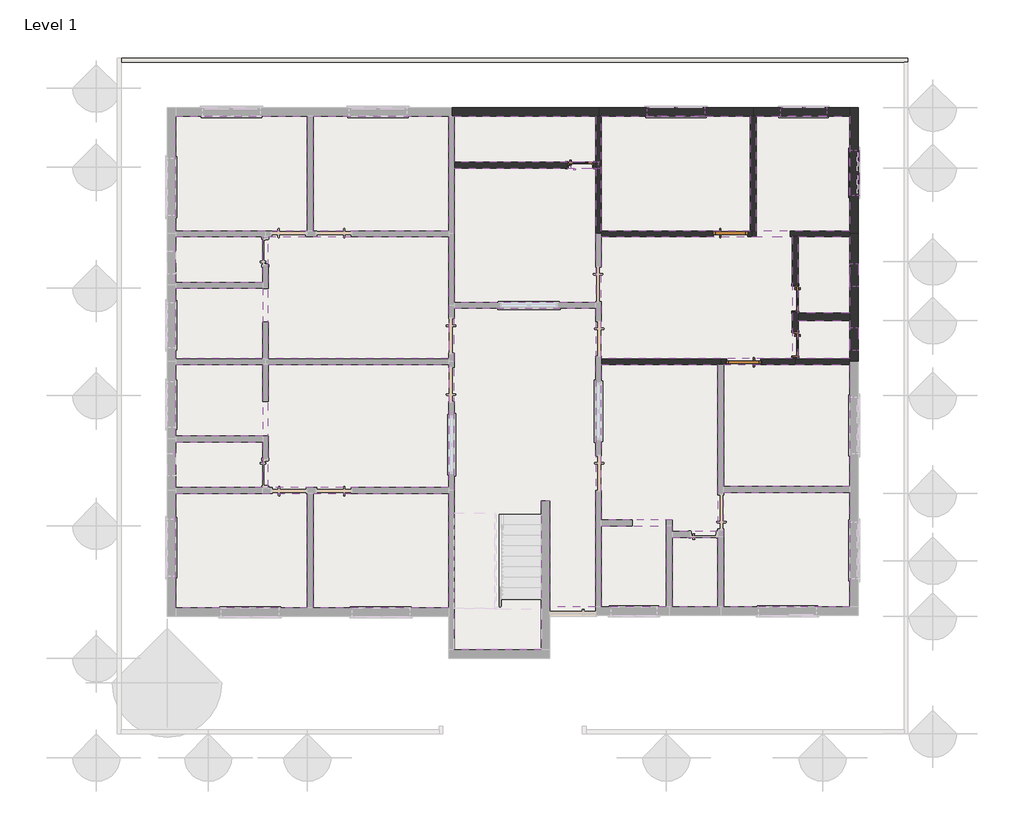
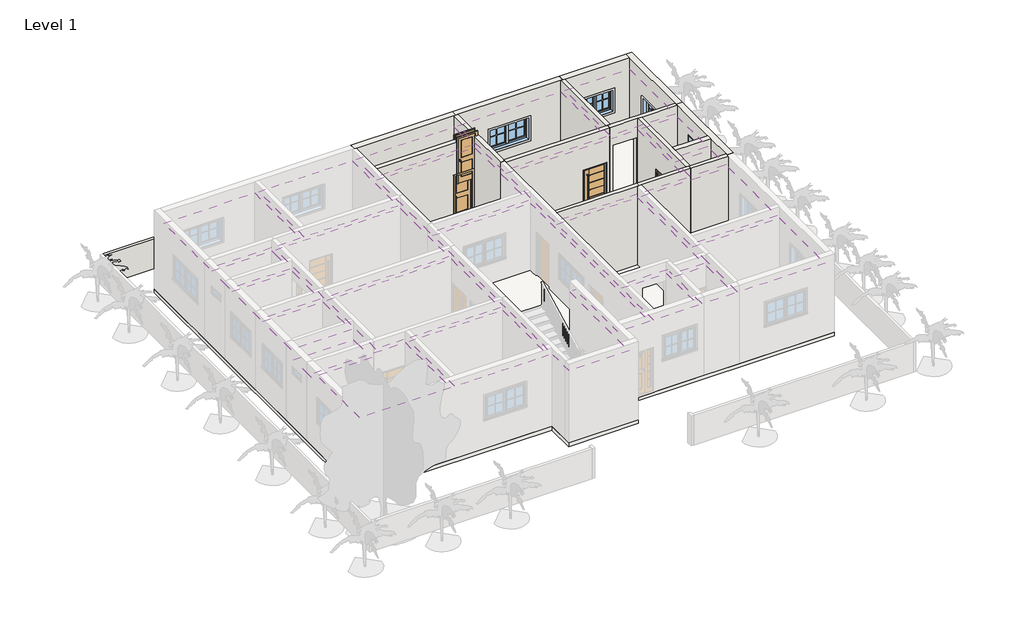
# One storey, part 3 of 5: 23 coverings, 16 walls, 6 doors, 5 windows, 1 slab.
"""IFC4 building model written with IfcOpenShell, lengths in millimetres."""

from ifc_helpers import new_model, si_unit, frame, origin, origin_with_axes, place, context, project, spatial, polyline, outline, extrude, faceted_brep, transform, mapped, element, save
from components import door_3_ad1505b7, m_door_interior_single_2_panel_wood_2_8c5b34de, door_57d9c04c, door_c5a180fb, fixed_2_d9cafb20, m_window_awning_double_horizontal_4_0c6a2509, m_window_awning_double_horizontal_5_7c720334

model = new_model("IFC4")

# Units and contexts
model_context = context("Model", 3, world=origin())
ifc_project = project(units=[si_unit("LENGTHUNIT", "METRE", prefix="MILLI")], contexts=[model_context])

# Site, building, storey
site = spatial("IfcSite", under=ifc_project)
building = spatial("IfcBuilding", under=site)
storey = spatial("IfcBuildingStorey", under=building, Name="Level 1", Elevation=0.0)

# Coverings
placement = place(None, origin())
element("IfcCovering", 1, ObjectType="2' x 4' ACT System", at=placement, inside=storey, context=model_context, shape_type="SweptSolid", body=[
    extrude(outline(polyline([(-22388.4847893, 20054.3922903), (-24776.0847893, 20054.3922903), (-24776.0847893, 23102.3922903), (-21270.8847893, 23102.3922903), (-21270.8847893, 20054.3922903), (-22388.4847893, 20054.3922903)])), frame((0.0, 0.0, 2743.2), z_axis=(0.0, 0.0, 1.0), x_axis=(1.0, 0.0, 0.0)), (0.0, 0.0, 1.0), 57.15),
])
element("IfcCovering", 2, ObjectType="2' x 4' ACT System", at=placement, inside=storey, context=model_context, shape_type="SweptSolid", body=[
    extrude(outline(polyline([(-21118.4847893, 23102.3922903), (-17511.6847893, 23102.3922903), (-17511.6847893, 20054.3922903), (-21118.4847893, 20054.3922903), (-21118.4847893, 23102.3922903)])), frame((0.0, 0.0, 2743.2), z_axis=(0.0, 0.0, 1.0), x_axis=(1.0, 0.0, 0.0)), (0.0, 0.0, 1.0), 57.15),
])
element("IfcCovering", 3, ObjectType="2' x 4' ACT System", at=placement, inside=storey, context=model_context, shape_type="SweptSolid", body=[
    extrude(outline(polyline([(-17511.6847893, 16650.7922903), (-22312.2847893, 16650.7922903), (-22312.2847893, 19901.9922903), (-17511.6847893, 19901.9922903), (-17511.6847893, 18073.1922903), (-17511.6847893, 16650.7922903)])), frame((0.0, 0.0, 2743.2), z_axis=(0.0, 0.0, 1.0), x_axis=(1.0, 0.0, 0.0)), (0.0, 0.0, 1.0), 57.15),
])
element("IfcCovering", 4, ObjectType="2' x 4' ACT System", at=placement, inside=storey, context=model_context, shape_type="SweptSolid", body=[
    extrude(outline(polyline([(-24776.0847893, 18682.7922903), (-24776.0847893, 19901.9922903), (-22464.6847893, 19901.9922903), (-22464.6847893, 18682.7922903), (-24776.0847893, 18682.7922903)])), frame((0.0, 0.0, 2743.2), z_axis=(0.0, 0.0, 1.0), x_axis=(1.0, 0.0, 0.0)), (0.0, 0.0, 1.0), 57.15),
])
element("IfcCovering", 5, ObjectType="2' x 4' ACT System", at=placement, inside=storey, context=model_context, shape_type="SweptSolid", body=[
    extrude(outline(polyline([(-22464.6847893, 18530.3922903), (-22464.6847893, 16650.7922903), (-24776.0847893, 16650.7922903), (-24776.0847893, 18530.3922903), (-22464.6847893, 18530.3922903)])), frame((0.0, 0.0, 2743.2), z_axis=(0.0, 0.0, 1.0), x_axis=(1.0, 0.0, 0.0)), (0.0, 0.0, 1.0), 57.15),
])
element("IfcCovering", 6, ObjectType="2' x 4' ACT System", at=placement, inside=storey, context=model_context, shape_type="SweptSolid", body=[
    extrude(outline(polyline([(-24776.0847893, 14593.3922903), (-24776.0847893, 16498.3922903), (-22464.6847893, 16498.3922903), (-22464.6847893, 14593.3922903), (-24776.0847893, 14593.3922903)])), frame((0.0, 0.0, 2743.2), z_axis=(0.0, 0.0, 1.0), x_axis=(1.0, 0.0, 0.0)), (0.0, 0.0, 1.0), 57.15),
])
element("IfcCovering", 7, ObjectType="2' x 4' ACT System", at=placement, inside=storey, context=model_context, shape_type="SweptSolid", body=[
    extrude(outline(polyline([(-22464.6847893, 13221.7922903), (-24776.0847893, 13221.7922903), (-24776.0847893, 14440.9922903), (-22464.6847893, 14440.9922903), (-22464.6847893, 13221.7922903)])), frame((0.0, 0.0, 2438.4), z_axis=(0.0, 0.0, 1.0), x_axis=(1.0, 0.0, 0.0)), (0.0, 0.0, 1.0), 57.15),
])
element("IfcCovering", 8, ObjectType="2' x 4' ACT System", at=placement, inside=storey, context=model_context, shape_type="SweptSolid", body=[
    extrude(outline(polyline([(-21270.8847893, 13069.3922903), (-21270.8847893, 10021.3922903), (-24776.0847893, 10021.3922903), (-24776.0847893, 13069.3922903), (-22477.3847893, 13069.3922903), (-21270.8847893, 13069.3922903)])), frame((0.0, 0.0, 2743.2), z_axis=(0.0, 0.0, 1.0), x_axis=(1.0, 0.0, 0.0)), (0.0, 0.0, 1.0), 57.15),
])
element("IfcCovering", 9, ObjectType="2' x 4' ACT System", at=placement, inside=storey, context=model_context, shape_type="SweptSolid", body=[
    extrude(outline(polyline([(-17511.6847893, 13221.7922903), (-22312.2847893, 13221.7922903), (-22312.2847893, 16498.3922903), (-17511.6847893, 16498.3922903), (-17511.6847893, 13221.7922903)])), frame((0.0, 0.0, 2743.2), z_axis=(0.0, 0.0, 1.0), x_axis=(1.0, 0.0, 0.0)), (0.0, 0.0, 1.0), 57.15),
])
element("IfcCovering", 10, ObjectType="2' x 4' ACT System", at=placement, inside=storey, context=model_context, shape_type="SweptSolid", body=[
    extrude(outline(polyline([(-17511.6847893, 10021.3922903), (-21118.4847893, 10021.3922903), (-21118.4847893, 13069.3922903), (-17511.6847893, 13069.3922903), (-17511.6847893, 10021.3922903)])), frame((0.0, 0.0, 2743.2), z_axis=(0.0, 0.0, 1.0), x_axis=(1.0, 0.0, 0.0)), (0.0, 0.0, 1.0), 57.15),
])
element("IfcCovering", 11, ObjectType="2' x 4' ACT System", at=placement, inside=storey, context=model_context, shape_type="SweptSolid", body=[
    extrude(outline(polyline([(-17359.2847893, 18149.3922903), (-17359.2847893, 19978.1922903), (-17359.2847893, 21730.7922903), (-13600.0847893, 21730.7922903), (-13600.0847893, 19978.1922903), (-13600.0847893, 18149.3922903), (-17359.2847893, 18149.3922903)])), frame((0.0, 0.0, 2743.2), z_axis=(0.0, 0.0, 1.0), x_axis=(1.0, 0.0, 0.0)), (0.0, 0.0, 1.0), 57.15),
])
element("IfcCovering", 12, ObjectType="2' x 4' ACT System", at=placement, inside=storey, context=model_context, shape_type="SweptSolid", body=[
    extrude(outline(polyline([(-13600.0847893, 21883.1922903), (-17359.2847893, 21883.1922903), (-17359.2847893, 23102.3922903), (-13600.0847893, 23102.3922903), (-13600.0847893, 21883.1922903)])), frame((0.0, 0.0, 2743.2), z_axis=(0.0, 0.0, 1.0), x_axis=(1.0, 0.0, 0.0)), (0.0, 0.0, 1.0), 57.15),
])
element("IfcCovering", 13, ObjectType="2' x 4' ACT System", at=placement, inside=storey, context=model_context, shape_type="SweptSolid", body=[
    extrude(outline(polyline([(-9485.2847893, 20054.3922903), (-13447.6847893, 20054.3922903), (-13447.6847893, 23102.3922903), (-9485.2847893, 23102.3922903), (-9485.2847893, 20054.3922903)])), frame((0.0, 0.0, 2743.2), z_axis=(0.0, 0.0, 1.0), x_axis=(1.0, 0.0, 0.0)), (0.0, 0.0, 1.0), 57.15),
])
element("IfcCovering", 14, ObjectType="2' x 4' ACT System", at=placement, inside=storey, context=model_context, shape_type="SweptSolid", body=[
    extrude(outline(polyline([(-9332.8847893, 20054.3922903), (-9332.8847893, 23102.3922903), (-6843.6847893, 23102.3922903), (-6843.6847893, 20054.3922903), (-9332.8847893, 20054.3922903)])), frame((0.0, 0.0, 2743.2), z_axis=(0.0, 0.0, 1.0), x_axis=(1.0, 0.0, 0.0)), (0.0, 0.0, 1.0), 57.15),
])
element("IfcCovering", 15, ObjectType="2' x 4' ACT System", at=placement, inside=storey, context=model_context, shape_type="SweptSolid", body=[
    extrude(outline(polyline([(-6843.6847893, 17869.9922903), (-8215.2847893, 17869.9922903), (-8215.2847893, 19901.9922903), (-6843.6847893, 19901.9922903), (-6843.6847893, 17869.9922903)])), frame((0.0, 0.0, 2743.2), z_axis=(0.0, 0.0, 1.0), x_axis=(1.0, 0.0, 0.0)), (0.0, 0.0, 1.0), 57.15),
])
element("IfcCovering", 16, ObjectType="2' x 4' ACT System", at=placement, inside=storey, context=model_context, shape_type="SweptSolid", body=[
    extrude(outline(polyline([(-13447.6847893, 16650.7922903), (-13447.6847893, 19901.9922903), (-9447.1847893, 19901.9922903), (-8367.6847893, 19901.9922903), (-8367.6847893, 16650.7922903), (-10272.6847893, 16650.7922903), (-13447.6847893, 16650.7922903)])), frame((0.0, 0.0, 2743.2), z_axis=(0.0, 0.0, 1.0), x_axis=(1.0, 0.0, 0.0)), (0.0, 0.0, 1.0), 57.15),
])
element("IfcCovering", 17, ObjectType="2' x 4' ACT System", at=placement, inside=storey, context=model_context, shape_type="SweptSolid", body=[
    extrude(outline(polyline([(-13447.6847893, 12358.1922903), (-13447.6847893, 16498.3922903), (-10348.8847893, 16498.3922903), (-10348.8847893, 12053.3922903), (-11568.0847893, 12053.3922903), (-11568.0847893, 12358.1922903), (-13447.6847893, 12358.1922903)])), frame((0.0, 0.0, 2743.2), z_axis=(0.0, 0.0, 1.0), x_axis=(1.0, 0.0, 0.0)), (0.0, 0.0, 1.0), 57.15),
])
element("IfcCovering", 18, ObjectType="2' x 4' ACT System", at=placement, inside=storey, context=model_context, shape_type="SweptSolid", body=[
    extrude(outline(polyline([(-6843.6847893, 16498.3922903), (-6843.6847893, 13247.1922903), (-10196.4847893, 13247.1922903), (-10196.4847893, 16498.3922903), (-8291.4847893, 16498.3922903), (-6843.6847893, 16498.3922903)])), frame((0.0, 0.0, 2743.2), z_axis=(0.0, 0.0, 1.0), x_axis=(1.0, 0.0, 0.0)), (0.0, 0.0, 1.0), 57.15),
])
element("IfcCovering", 19, ObjectType="2' x 4' ACT System", at=placement, inside=storey, context=model_context, shape_type="SweptSolid", body=[
    extrude(outline(polyline([(-6843.6847893, 13094.7922903), (-6843.6847893, 10046.7922903), (-10196.4847893, 10046.7922903), (-10196.4847893, 11913.6922903), (-10196.4847893, 13094.7922903), (-6843.6847893, 13094.7922903)])), frame((0.0, 0.0, 2743.2), z_axis=(0.0, 0.0, 1.0), x_axis=(1.0, 0.0, 0.0)), (0.0, 0.0, 1.0), 57.15),
])
element("IfcCovering", 20, ObjectType="2' x 4' ACT System", at=placement, inside=storey, context=model_context, shape_type="SweptSolid", body=[
    extrude(outline(polyline([(-11568.0847893, 10046.7922903), (-11568.0847893, 11900.9922903), (-10348.8847893, 11900.9922903), (-10348.8847893, 10046.7922903), (-11568.0847893, 10046.7922903)])), frame((0.0, 0.0, 2743.2), z_axis=(0.0, 0.0, 1.0), x_axis=(1.0, 0.0, 0.0)), (0.0, 0.0, 1.0), 57.15),
])
element("IfcCovering", 21, ObjectType="2' x 4' ACT System", at=placement, inside=storey, context=model_context, shape_type="SweptSolid", body=[
    extrude(outline(polyline([(-13447.6847893, 10046.7922903), (-13447.6847893, 12205.7922903), (-11720.4847893, 12205.7922903), (-11720.4847893, 10046.7922903), (-13447.6847893, 10046.7922903)])), frame((0.0, 0.0, 2743.2), z_axis=(0.0, 0.0, 1.0), x_axis=(1.0, 0.0, 0.0)), (0.0, 0.0, 1.0), 57.15),
])
element("IfcCovering", 22, ObjectType="2' x 4' ACT System", at=placement, inside=storey, context=model_context, shape_type="SweptSolid", body=[
    extrude(outline(polyline([(-6843.6847893, 16650.7922903), (-8215.2847893, 16650.7922903), (-8215.2847893, 17666.7922903), (-6843.6847893, 17666.7922903), (-6843.6847893, 16650.7922903)])), frame((0.0, 0.0, 2743.2), z_axis=(0.0, 0.0, 1.0), x_axis=(1.0, 0.0, 0.0)), (0.0, 0.0, 1.0), 57.15),
])
element("IfcCovering", 23, ObjectType="2' x 4' ACT System", at=placement, inside=storey, context=model_context, shape_type="SweptSolid", body=[
    extrude(outline(polyline([(-15047.8847893, 12866.1922903), (-15047.8847893, 8903.7922903), (-17359.2847893, 8903.7922903), (-17359.2847893, 13145.5922903), (-17359.2847893, 16574.5922903), (-17359.2847893, 17996.9922903), (-13600.0847893, 17996.9922903), (-13600.0847893, 10046.7922903), (-14819.2847893, 10046.7922903), (-14819.2847893, 12866.1922903), (-15047.8847893, 12866.1922903)])), frame((0.0, 0.0, 2743.2), z_axis=(0.0, 0.0, 1.0), x_axis=(1.0, 0.0, 0.0)), (0.0, 0.0, 1.0), 57.15),
])

# Doors
door_3_shape = door_3_ad1505b7(model_context)
element("IfcDoor", 24, ObjectType="3'", at=placement, inside=storey, context=model_context, shape_type="MappedRepresentation", body=[
    mapped(door_3_shape, transform((-10018.6847893, 19978.1922903, 0.0), x_axis=(1.0, 0.0, 0.0), y_axis=(0.0, 1.0, 0.0), z_axis=(0.0, 0.0, 1.0))),
])
element("IfcDoor", 25, ObjectType="3'", at=placement, inside=storey, context=model_context, shape_type="MappedRepresentation", body=[
    mapped(door_3_shape, transform((-9663.0847893, 16574.5922903, 0.0), x_axis=(-1.0, 0.0, 0.0), y_axis=(0.0, -1.0, 0.0), z_axis=(0.0, 0.0, 1.0))),
])
m_door_interior_single_2_panel_wood_2_shape = m_door_interior_single_2_panel_wood_2_8c5b34de(model_context)
element("IfcDoor", 26, ObjectType="M_Door-Interior-Single-2_Panel-Wood : 2'", at=placement, inside=storey, context=model_context, shape_type="MappedRepresentation", body=[
    mapped(m_door_interior_single_2_panel_wood_2_shape, transform((-8288.3097893, 17031.7922903, 0.0), x_axis=(0.0, -1.0, 0.0), y_axis=(1.0, 0.0, 0.0), z_axis=(0.0, 0.0, 1.0))),
])
door_shape = door_57d9c04c(model_context)
element("IfcDoor", 27, ObjectType="M_Door-Interior-Single-2_Panel-Wood : 2'2\"", at=placement, inside=storey, context=model_context, shape_type="MappedRepresentation", body=[
    mapped(door_shape, transform((-14006.4847893, 21810.1672903, 0.0), x_axis=(1.0, 0.0, 0.0), y_axis=(0.0, 1.0, 0.0), z_axis=(0.0, 0.0, 1.0))),
])
element("IfcDoor", 28, ObjectType="M_Door-Interior-Single-2_Panel-Wood : 2'2\"", at=placement, inside=storey, context=model_context, shape_type="MappedRepresentation", body=[
    mapped(door_shape, transform((-8288.3097893, 18250.9922903, 0.0), x_axis=(0.0, -1.0, 0.0), y_axis=(1.0, 0.0, 0.0), z_axis=(0.0, 0.0, 1.0))),
])
door_2_shape = door_c5a180fb(model_context)
element("IfcDoor", 29, ObjectType="M_Door-Interior-Single-2_Panel-Wood : 2'2\"", at=placement, inside=storey, context=model_context, shape_type="MappedRepresentation", body=[
    mapped(door_2_shape, transform((-13892.1847893, 21803.8172903, 1493.7515697), x_axis=(1.0, 0.0, 0.0), y_axis=(0.0, 1.0, 0.0), z_axis=(0.0, 0.0, 1.0))),
])

# Slab
element("IfcSlab", 30, ObjectType="Generic - 6\"", at=placement, inside=storey, context=model_context, shape_type="SweptSolid", body=[
    extrude(outline(polyline([(-25004.6847893, 9792.7922903), (-25004.6847893, 23330.9922903), (-6615.0847893, 23330.9922903), (-6615.0847893, 9818.1922903), (-14819.2847893, 9818.1922903), (-14819.2847893, 8675.1922903), (-17511.6847893, 8675.1922903), (-17511.6847893, 9792.7922903), (-25004.6847893, 9792.7922903)])), frame((0.0, 0.0, -152.4), z_axis=(0.0, 0.0, 1.0), x_axis=(1.0, 0.0, 0.0)), (0.0, 0.0, 1.0), 152.4),
])

# Walls
element("IfcWall", 31, ObjectType="Generic - 4\"", at=placement, inside=storey, context=model_context, shape_type="Brep", body=[
    faceted_brep([(-26223.8847893, 24550.1922903, -152.4), (-5395.8847893, 24550.1922903, -152.4), (-5294.2847893, 24550.1922903, -152.4), (-5294.2847893, 24550.1922903, 1066.8), (-5395.8847893, 24550.1922903, 1066.8), (-26223.8847893, 24550.1922903, 1066.8), (-26223.8847893, 24651.7922903, -152.4), (-26223.8847893, 24651.7922903, 1066.8), (-5294.2847893, 24651.7922903, 1066.8), (-5294.2847893, 24651.7922903, -152.4)], [[[0, 1, 2, 3, 4, 5]], [[6, 7, 8, 9]], [[2, 1, 0, 6, 9]], [[5, 4, 3, 8, 7]], [[0, 5, 7, 6]], [[3, 2, 9, 8]]]),
])
element("IfcWall", 32, ObjectType="Generic - 6\"", at=placement, inside=storey, context=model_context, shape_type="Brep", body=[
    faceted_brep([(-13600.0847893, 23102.3922903, 0.0), (-13600.0847893, 21883.1922903, 0.0), (-13600.0847893, 21730.7922903, 0.0), (-13600.0847893, 19978.1922903, 0.0), (-13600.0847893, 19978.1922903, 3200.4), (-13600.0847893, 21730.7922903, 3200.4), (-13600.0847893, 21730.7922903, 1493.7515697), (-13600.0847893, 21883.1922903, 1493.7515697), (-13600.0847893, 21883.1922903, 3200.4), (-13600.0847893, 23102.3922903, 3200.4), (-13447.6847893, 19978.1922903, 0.0), (-13447.6847893, 20054.3922903, 0.0), (-13447.6847893, 23102.3922903, 0.0), (-13447.6847893, 23102.3922903, 3200.4), (-13447.6847893, 20054.3922903, 3200.4), (-13447.6847893, 19978.1922903, 3200.4), (-13523.8847893, 23102.3922903, 0.0), (-13523.8847893, 23102.3922903, 3200.4), (-13536.9847893, 21883.1922903, 3200.4), (-13536.9847893, 21730.7922903, 3200.4), (-13536.9847893, 21730.7922903, 1493.7515697), (-13536.9847893, 21883.1922903, 1493.7515697)], [[[0, 1, 2, 3, 4, 5, 6, 7, 8, 9]], [[10, 11, 12, 13, 14, 15]], [[3, 2, 1, 0, 16, 12, 11, 10]], [[4, 3, 10, 15]], [[15, 14, 13, 17, 9, 8, 18, 19, 5, 4]], [[0, 9, 17, 13, 12, 16]], [[20, 6, 5, 19]], [[21, 18, 8, 7]], [[20, 21, 7, 6]], [[21, 20, 19, 18]]]),
])
element("IfcWall", 33, ObjectType="Generic - 6\"", at=placement, inside=storey, context=model_context, shape_type="SweptSolid", body=[
    extrude(outline(polyline([(3200.4, -17359.2847893), (0.0, -17359.2847893), (0.0, -14361.6847893), (1853.8, -14361.6847893), (1853.8, -14247.3847893), (3200.4, -14247.3847893), (3200.4, -17359.2847893)])), frame((0.0, 21730.7922903, 0.0), z_axis=(0.0, 1.0, 0.0), x_axis=(0.0, 0.0, 1.0)), (0.0, 0.0, 1.0), 152.4),
    extrude(outline(polyline([(-13600.0847893, 21883.1922903), (-13600.0847893, 21730.7922903), (-13651.2847893, 21730.7922903), (-13651.2847893, 21883.1922903), (-13600.0847893, 21883.1922903)])), origin_with_axes(), (0.0, 0.0, 1.0), 1493.7515697),
])
element("IfcWall", 34, ObjectType="Generic - 6\"", at=placement, inside=storey, context=model_context, shape_type="Brep", body=[
    faceted_brep([(-9447.1847893, 19901.9922903, 0.0), (-9447.1847893, 19901.9922903, 3200.4), (-13447.6847893, 19901.9922903, 3200.4), (-13447.6847893, 19901.9922903, 0.0), (-10475.8847893, 19901.9922903, 0.0), (-10475.8847893, 19901.9922903, 1828.8), (-9561.4847893, 19901.9922903, 1828.8), (-9561.4847893, 19901.9922903, 0.0), (-9447.1847893, 20054.3922903, 3200.4), (-9447.1847893, 20054.3922903, 0.0), (-9485.2847893, 20054.3922903, 0.0), (-9561.4847893, 20054.3922903, 0.0), (-9561.4847893, 20054.3922903, 1828.8), (-10475.8847893, 20054.3922903, 1828.8), (-10475.8847893, 20054.3922903, 0.0), (-13447.6847893, 20054.3922903, 0.0), (-13447.6847893, 20054.3922903, 3200.4), (-9485.2847893, 20054.3922903, 3200.4), (-13447.6847893, 19978.1922903, 0.0), (-10475.8847893, 20034.3922903, 0.0), (-10490.8847893, 20034.3922903, 0.0), (-10490.8847893, 19957.3922903, 0.0), (-10475.8847893, 19957.3922903, 0.0), (-9561.4847893, 19957.3922903, 0.0), (-9546.4847893, 19957.3922903, 0.0), (-9546.4847893, 20034.3922903, 0.0), (-9561.4847893, 20034.3922903, 0.0), (-13447.6847893, 19978.1922903, 3200.4), (-9561.4847893, 20034.3922903, 1828.8), (-10475.8847893, 20034.3922903, 1828.8), (-10475.8847893, 19957.3922903, 1828.8), (-9561.4847893, 19957.3922903, 1828.8), (-10490.8847893, 20034.3922903, 1843.8), (-9546.4847893, 20034.3922903, 1843.8), (-9546.4847893, 19957.3922903, 1843.8), (-10490.8847893, 19957.3922903, 1843.8)], [[[0, 1, 2, 3, 4, 5, 6, 7]], [[8, 9, 10, 11, 12, 13, 14, 15, 16, 17]], [[3, 18, 15, 14, 19, 20, 21, 22, 4]], [[9, 0, 7, 23, 24, 25, 26, 11, 10]], [[1, 0, 9, 8]], [[2, 1, 8, 17, 16, 27]], [[3, 2, 27, 16, 15, 18]], [[12, 28, 29, 13]], [[5, 30, 31, 6]], [[28, 12, 11, 26]], [[6, 31, 23, 7]], [[13, 29, 19, 14]], [[30, 5, 4, 22]], [[32, 33, 34, 35]], [[34, 33, 25, 24]], [[31, 30, 22, 21, 35, 34, 24, 23]], [[32, 35, 21, 20]], [[29, 28, 26, 25, 33, 32, 20, 19]]]),
])
element("IfcWall", 35, ObjectType="Generic - 6\"", at=placement, inside=storey, context=model_context, shape_type="Brep", body=[
    faceted_brep([(-9485.2847893, 23102.3922903, 0.0), (-9485.2847893, 20054.3922903, 0.0), (-9485.2847893, 20054.3922903, 3200.4), (-9485.2847893, 23102.3922903, 3200.4), (-9332.8847893, 23102.3922903, 0.0), (-9332.8847893, 23102.3922903, 3200.4), (-9332.8847893, 20054.3922903, 3200.4), (-9332.8847893, 20054.3922903, 2438.4), (-9332.8847893, 20054.3922903, 0.0), (-9409.0847893, 23102.3922903, 0.0), (-9447.1847893, 20054.3922903, 0.0), (-9447.1847893, 20054.3922903, 3200.4), (-9409.0847893, 23102.3922903, 3200.4)], [[[0, 1, 2, 3]], [[4, 5, 6, 7, 8]], [[1, 0, 9, 4, 8, 10]], [[3, 2, 11, 6, 5, 12]], [[0, 3, 12, 5, 4, 9]], [[2, 1, 10, 8, 7, 6, 11]]]),
])
element("IfcWall", 36, ObjectType="Generic - 6\"", at=placement, inside=storey, context=model_context, shape_type="Brep", body=[
    faceted_brep([(-8367.6847893, 16650.7922903, 3200.4), (-8367.6847893, 19901.9922903, 3200.4), (-8367.6847893, 19901.9922903, 0.0), (-8367.6847893, 18606.1922903, 0.0), (-8367.6847893, 18606.1922903, 1853.8), (-8367.6847893, 17895.7922903, 1853.8), (-8367.6847893, 17895.7922903, 0.0), (-8367.6847893, 17361.5922903, 0.0), (-8367.6847893, 17361.5922903, 1853.8), (-8367.6847893, 16701.9922903, 1853.8), (-8367.6847893, 16701.9922903, 0.0), (-8367.6847893, 16650.7922903, 0.0), (-8215.2847893, 19901.9922903, 3200.4), (-8215.2847893, 17869.9922903, 3200.4), (-8215.2847893, 17666.7922903, 3200.4), (-8215.2847893, 16650.7922903, 3200.4), (-8215.2847893, 16650.7922903, 0.0), (-8215.2847893, 16701.9922903, 0.0), (-8215.2847893, 16701.9922903, 1853.8), (-8215.2847893, 17361.5922903, 1853.8), (-8215.2847893, 17361.5922903, 0.0), (-8215.2847893, 17666.7922903, 0.0), (-8215.2847893, 17869.9922903, 0.0), (-8215.2847893, 17895.7922903, 0.0), (-8215.2847893, 17895.7922903, 1853.8), (-8215.2847893, 18606.1922903, 1853.8), (-8215.2847893, 18606.1922903, 0.0), (-8215.2847893, 19901.9922903, 0.0), (-8291.4847893, 16650.7922903, 0.0), (-8291.4847893, 16650.7922903, 3200.4)], [[[0, 1, 2, 3, 4, 5, 6, 7, 8, 9, 10, 11]], [[12, 13, 14, 15, 16, 17, 18, 19, 20, 21, 22, 23, 24, 25, 26, 27]], [[2, 27, 26, 3]], [[16, 28, 11, 10, 17]], [[20, 7, 6, 23, 22, 21]], [[1, 0, 29, 15, 14, 13, 12]], [[2, 1, 12, 27]], [[0, 11, 28, 16, 15, 29]], [[9, 18, 17, 10]], [[18, 9, 8, 19]], [[19, 8, 7, 20]], [[5, 24, 23, 6]], [[24, 5, 4, 25]], [[25, 4, 3, 26]]]),
])
element("IfcWall", 37, ObjectType="Generic - 6\"", at=placement, inside=storey, context=model_context, shape_type="Brep", body=[
    faceted_brep([(-13447.6847893, 16498.3922903, 0.0), (-10348.8847893, 16498.3922903, 0.0), (-10272.6847893, 16498.3922903, 0.0), (-10272.6847893, 16498.3922903, 3200.4), (-10348.8847893, 16498.3922903, 3200.4), (-13447.6847893, 16498.3922903, 3200.4), (-13447.6847893, 16650.7922903, 0.0), (-13447.6847893, 16650.7922903, 3200.4), (-10272.6847893, 16650.7922903, 3200.4), (-10272.6847893, 16650.7922903, 0.0)], [[[0, 1, 2, 3, 4, 5]], [[6, 7, 8, 9]], [[2, 1, 0, 6, 9]], [[3, 2, 9, 8]], [[5, 4, 3, 8, 7]], [[0, 5, 7, 6]]]),
])
element("IfcWall", 38, ObjectType="Generic - 6\"", at=placement, inside=storey, context=model_context, shape_type="Brep", body=[
    faceted_brep([(-8291.4847893, 16498.3922903, 0.0), (-8291.4847893, 16498.3922903, 3200.4), (-10196.4847893, 16498.3922903, 3200.4), (-10272.6847893, 16498.3922903, 3200.4), (-10272.6847893, 16498.3922903, 0.0), (-10196.4847893, 16498.3922903, 0.0), (-10120.2847893, 16498.3922903, 0.0), (-10120.2847893, 16498.3922903, 1828.8), (-9205.8847893, 16498.3922903, 1828.8), (-9205.8847893, 16498.3922903, 0.0), (-8291.4847893, 16650.7922903, 3200.4), (-8291.4847893, 16650.7922903, 0.0), (-8367.6847893, 16650.7922903, 0.0), (-9205.8847893, 16650.7922903, 0.0), (-9205.8847893, 16650.7922903, 1828.8), (-10120.2847893, 16650.7922903, 1828.8), (-10120.2847893, 16650.7922903, 0.0), (-10272.6847893, 16650.7922903, 0.0), (-10272.6847893, 16650.7922903, 3200.4), (-8367.6847893, 16650.7922903, 3200.4), (-10120.2847893, 16595.3922903, 0.0), (-10135.2847893, 16595.3922903, 0.0), (-10135.2847893, 16518.3922903, 0.0), (-10120.2847893, 16518.3922903, 0.0), (-9205.8847893, 16518.3922903, 0.0), (-9190.8847893, 16518.3922903, 0.0), (-9190.8847893, 16595.3922903, 0.0), (-9205.8847893, 16595.3922903, 0.0), (-9205.8847893, 16595.3922903, 1828.8), (-10120.2847893, 16595.3922903, 1828.8), (-10120.2847893, 16518.3922903, 1828.8), (-9205.8847893, 16518.3922903, 1828.8), (-9190.8847893, 16518.3922903, 1843.8), (-10135.2847893, 16518.3922903, 1843.8), (-10135.2847893, 16595.3922903, 1843.8), (-9190.8847893, 16595.3922903, 1843.8)], [[[0, 1, 2, 3, 4, 5, 6, 7, 8, 9]], [[10, 11, 12, 13, 14, 15, 16, 17, 18, 19]], [[4, 17, 16, 20, 21, 22, 23, 6, 5]], [[11, 0, 9, 24, 25, 26, 27, 13, 12]], [[1, 0, 11, 10]], [[3, 2, 1, 10, 19, 18]], [[4, 3, 18, 17]], [[14, 28, 29, 15]], [[7, 30, 31, 8]], [[15, 29, 20, 16]], [[30, 7, 6, 23]], [[28, 14, 13, 27]], [[8, 31, 24, 9]], [[32, 33, 34, 35]], [[34, 33, 22, 21]], [[29, 28, 27, 26, 35, 34, 21, 20]], [[32, 35, 26, 25]], [[31, 30, 23, 22, 33, 32, 25, 24]]]),
])
element("IfcWall", 39, ObjectType="Generic - 6\"", at=placement, inside=storey, context=model_context, shape_type="Brep", body=[
    faceted_brep([(-6843.6847893, 19901.9922903, 0.0), (-6843.6847893, 19901.9922903, 3200.4), (-8215.2847893, 19901.9922903, 3200.4), (-8367.6847893, 19901.9922903, 3200.4), (-9447.1847893, 19901.9922903, 3200.4), (-9447.1847893, 19901.9922903, 0.0), (-9332.8847893, 19901.9922903, 0.0), (-9332.8847893, 19901.9922903, 2438.4), (-8430.9142678, 19901.9922903, 2438.4), (-8430.9142678, 19901.9922903, 0.0), (-8367.6847893, 19901.9922903, 0.0), (-8215.2847893, 19901.9922903, 0.0), (-6843.6847893, 20054.3922903, 3200.4), (-6843.6847893, 20054.3922903, 0.0), (-8430.9142678, 20054.3922903, 0.0), (-8430.9142678, 20054.3922903, 2438.4), (-9332.8847893, 20054.3922903, 2438.4), (-9332.8847893, 20054.3922903, 0.0), (-9447.1847893, 20054.3922903, 0.0), (-9447.1847893, 20054.3922903, 3200.4), (-9332.8847893, 20054.3922903, 3200.4), (-6843.6847893, 19978.1922903, 0.0), (-6843.6847893, 19978.1922903, 3200.4)], [[[0, 1, 2, 3, 4, 5, 6, 7, 8, 9, 10, 11]], [[12, 13, 14, 15, 16, 17, 18, 19, 20]], [[13, 21, 0, 11, 10, 9, 14]], [[5, 18, 17, 6]], [[4, 3, 2, 1, 22, 12, 20, 19]], [[5, 4, 19, 18]], [[1, 0, 21, 13, 12, 22]], [[7, 16, 15, 8]], [[16, 7, 6, 17]], [[8, 15, 14, 9]]]),
])
element("IfcWall", 40, ObjectType="Generic - 6\"", at=placement, inside=storey, context=model_context, shape_type="Brep", body=[
    faceted_brep([(-8291.4847893, 16498.3922903, 0.0), (-6843.6847893, 16498.3922903, 0.0), (-6843.6847893, 16498.3922903, 3200.4), (-8291.4847893, 16498.3922903, 3200.4), (-8291.4847893, 16650.7922903, 0.0), (-8291.4847893, 16650.7922903, 3200.4), (-8215.2847893, 16650.7922903, 3200.4), (-6843.6847893, 16650.7922903, 3200.4), (-6843.6847893, 16650.7922903, 0.0), (-8215.2847893, 16650.7922903, 0.0), (-6843.6847893, 16574.5922903, 0.0), (-6843.6847893, 16574.5922903, 3200.4)], [[[0, 1, 2, 3]], [[4, 5, 6, 7, 8, 9]], [[1, 0, 4, 9, 8, 10]], [[3, 2, 11, 7, 6, 5]], [[0, 3, 5, 4]], [[2, 1, 10, 8, 7, 11]]]),
])
element("IfcWall", 41, ObjectType="Generic - 8\"", at=placement, inside=storey, context=model_context, shape_type="SweptSolid", body=[
    extrude(outline(polyline([(-6843.6847893, 17666.7922903), (-8215.2847893, 17666.7922903), (-8215.2847893, 17869.9922903), (-6843.6847893, 17869.9922903), (-6843.6847893, 17666.7922903)])), origin_with_axes(), (0.0, 0.0, 1.0), 3200.4),
])
element("IfcWall", 42, ObjectType="Generic - 9\"", at=placement, inside=storey, context=model_context, shape_type="Brep", body=[
    faceted_brep([(-6843.6847893, 23330.9922903, 0.0), (-9409.0847893, 23330.9922903, 0.0), (-9409.0847893, 23330.9922903, 3200.4), (-6843.6847893, 23330.9922903, 3200.4), (-7459.6347893, 23330.9922903, 2133.6), (-8678.8347893, 23330.9922903, 2133.6), (-8678.8347893, 23330.9922903, 1219.2), (-7459.6347893, 23330.9922903, 1219.2), (-6843.6847893, 23102.3922903, 0.0), (-6843.6847893, 23102.3922903, 3200.4), (-9332.8847893, 23102.3922903, 3200.4), (-9409.0847893, 23102.3922903, 3200.4), (-9409.0847893, 23102.3922903, 0.0), (-9332.8847893, 23102.3922903, 0.0), (-7459.6347893, 23102.3922903, 2133.6), (-7459.6347893, 23102.3922903, 1219.2), (-8678.8347893, 23102.3922903, 1219.2), (-8678.8347893, 23102.3922903, 2133.6)], [[[0, 1, 2, 3], [4, 5, 6, 7]], [[8, 9, 10, 11, 12, 13], [14, 15, 16, 17]], [[1, 0, 8, 13, 12]], [[2, 1, 12, 11]], [[3, 2, 11, 10, 9]], [[0, 3, 9, 8]], [[15, 14, 4, 7]], [[16, 15, 7, 6]], [[17, 16, 6, 5]], [[14, 17, 5, 4]]]),
])
element("IfcWall", 43, ObjectType="Generic - 9\"", at=placement, inside=storey, context=model_context, shape_type="Brep", body=[
    faceted_brep([(-13523.8847893, 23330.9922903, 0.0), (-17435.4847893, 23330.9922903, 0.0), (-17435.4847893, 23330.9922903, 3200.4), (-13523.8847893, 23330.9922903, 3200.4), (-13523.8847893, 23102.3922903, 0.0), (-13523.8847893, 23102.3922903, 3200.4), (-13600.0847893, 23102.3922903, 3200.4), (-17359.2847893, 23102.3922903, 3200.4), (-17435.4847893, 23102.3922903, 3200.4), (-17435.4847893, 23102.3922903, 0.0), (-17359.2847893, 23102.3922903, 0.0), (-13600.0847893, 23102.3922903, 0.0)], [[[0, 1, 2, 3]], [[4, 5, 6, 7, 8, 9, 10, 11]], [[1, 0, 4, 11, 10, 9]], [[2, 1, 9, 8]], [[3, 2, 8, 7, 6, 5]], [[0, 3, 5, 4]]]),
])
element("IfcWall", 44, ObjectType="Generic - 9\"", at=placement, inside=storey, context=model_context, shape_type="Brep", body=[
    faceted_brep([(-9409.0847893, 23330.9922903, 0.0), (-13523.8847893, 23330.9922903, 0.0), (-13523.8847893, 23330.9922903, 3200.4), (-9409.0847893, 23330.9922903, 3200.4), (-10704.4847893, 23330.9922903, 2133.5570313), (-12228.4847893, 23330.9922903, 2133.5570313), (-12228.4847893, 23330.9922903, 1219.1570313), (-10704.4847893, 23330.9922903, 1219.1570313), (-9409.0847893, 23102.3922903, 0.0), (-9409.0847893, 23102.3922903, 3200.4), (-9485.2847893, 23102.3922903, 3200.4), (-13447.6847893, 23102.3922903, 3200.4), (-13523.8847893, 23102.3922903, 3200.4), (-13523.8847893, 23102.3922903, 0.0), (-13447.6847893, 23102.3922903, 0.0), (-9485.2847893, 23102.3922903, 0.0), (-10704.4847893, 23102.3922903, 2133.5570313), (-10704.4847893, 23102.3922903, 1219.1570313), (-12228.4847893, 23102.3922903, 1219.1570313), (-12228.4847893, 23102.3922903, 2133.5570313)], [[[0, 1, 2, 3], [4, 5, 6, 7]], [[8, 9, 10, 11, 12, 13, 14, 15], [16, 17, 18, 19]], [[1, 0, 8, 15, 14, 13]], [[2, 1, 13, 12]], [[3, 2, 12, 11, 10, 9]], [[0, 3, 9, 8]], [[16, 19, 5, 4]], [[19, 18, 6, 5]], [[18, 17, 7, 6]], [[17, 16, 4, 7]]]),
])
element("IfcWall", 45, ObjectType="Generic - 9\"", at=placement, inside=storey, context=model_context, shape_type="Brep", body=[
    faceted_brep([(-6615.0847893, 19978.1922903, 0.0), (-6615.0847893, 23330.9922903, 0.0), (-6615.0847893, 23330.9922903, 3200.4), (-6615.0847893, 19978.1922903, 3200.4), (-6615.0847893, 20987.8422903, 2133.6), (-6615.0847893, 22207.0422903, 2133.6), (-6615.0847893, 22207.0422903, 1219.2), (-6615.0847893, 20987.8422903, 1219.2), (-6843.6847893, 19978.1922903, 0.0), (-6843.6847893, 19978.1922903, 3200.4), (-6843.6847893, 20054.3922903, 3200.4), (-6843.6847893, 23102.3922903, 3200.4), (-6843.6847893, 23330.9922903, 3200.4), (-6843.6847893, 23330.9922903, 0.0), (-6843.6847893, 23102.3922903, 0.0), (-6843.6847893, 20054.3922903, 0.0), (-6843.6847893, 20987.8422903, 2133.6), (-6843.6847893, 20987.8422903, 1219.2), (-6843.6847893, 22207.0422903, 1219.2), (-6843.6847893, 22207.0422903, 2133.6)], [[[0, 1, 2, 3], [4, 5, 6, 7]], [[8, 9, 10, 11, 12, 13, 14, 15], [16, 17, 18, 19]], [[1, 0, 8, 15, 14, 13]], [[3, 2, 12, 11, 10, 9]], [[0, 3, 9, 8]], [[2, 1, 13, 12]], [[16, 19, 5, 4]], [[19, 18, 6, 5]], [[18, 17, 7, 6]], [[17, 16, 4, 7]]]),
])
element("IfcWall", 46, ObjectType="Generic - 9\"", at=placement, inside=storey, context=model_context, shape_type="Brep", body=[
    faceted_brep([(-6615.0847893, 16574.5922903, 0.0), (-6615.0847893, 19978.1922903, 0.0), (-6615.0847893, 19978.1922903, 3200.4), (-6615.0847893, 16574.5922903, 3200.4), (-6615.0847893, 16866.6922903, 2438.4), (-6615.0847893, 17476.2922903, 2438.4), (-6615.0847893, 17476.2922903, 2133.6), (-6615.0847893, 16866.6922903, 2133.6), (-6615.0847893, 18568.4922903, 2438.4), (-6615.0847893, 19178.0922903, 2438.4), (-6615.0847893, 19178.0922903, 2133.6), (-6615.0847893, 18568.4922903, 2133.6), (-6843.6847893, 16574.5922903, 0.0), (-6843.6847893, 16574.5922903, 3200.4), (-6843.6847893, 16650.7922903, 3200.4), (-6843.6847893, 17666.7922903, 3200.4), (-6843.6847893, 17869.9922903, 3200.4), (-6843.6847893, 19901.9922903, 3200.4), (-6843.6847893, 19978.1922903, 3200.4), (-6843.6847893, 19978.1922903, 0.0), (-6843.6847893, 19901.9922903, 0.0), (-6843.6847893, 17869.9922903, 0.0), (-6843.6847893, 17666.7922903, 0.0), (-6843.6847893, 16650.7922903, 0.0), (-6843.6847893, 16866.6922903, 2438.4), (-6843.6847893, 16866.6922903, 2133.6), (-6843.6847893, 17476.2922903, 2133.6), (-6843.6847893, 17476.2922903, 2438.4), (-6843.6847893, 18568.4922903, 2438.4), (-6843.6847893, 18568.4922903, 2133.6), (-6843.6847893, 19178.0922903, 2133.6), (-6843.6847893, 19178.0922903, 2438.4)], [[[0, 1, 2, 3], [4, 5, 6, 7], [8, 9, 10, 11]], [[12, 13, 14, 15, 16, 17, 18, 19, 20, 21, 22, 23], [24, 25, 26, 27], [28, 29, 30, 31]], [[1, 0, 12, 23, 22, 21, 20, 19]], [[2, 1, 19, 18]], [[3, 2, 18, 17, 16, 15, 14, 13]], [[0, 3, 13, 12]], [[24, 27, 5, 4]], [[27, 26, 6, 5]], [[26, 25, 7, 6]], [[25, 24, 4, 7]], [[28, 31, 9, 8]], [[31, 30, 10, 9]], [[30, 29, 11, 10]], [[29, 28, 8, 11]]]),
])

# Windows
fixed_2_shape = fixed_2_d9cafb20(model_context)
element("IfcWindow", 47, ObjectType="Fixed : 2'", at=placement, inside=storey, context=model_context, shape_type="MappedRepresentation", body=[
    mapped(fixed_2_shape, transform((-6729.3847893, 17133.3922903, 0.0), x_axis=(0.0, -1.0, 0.0), y_axis=(1.0, 0.0, 0.0), z_axis=(0.0, 0.0, 1.0))),
])
element("IfcWindow", 48, ObjectType="Fixed : 2'", at=placement, inside=storey, context=model_context, shape_type="MappedRepresentation", body=[
    mapped(fixed_2_shape, transform((-6729.3847893, 18835.1922903, 0.0), x_axis=(0.0, -1.0, 0.0), y_axis=(1.0, 0.0, 0.0), z_axis=(0.0, 0.0, 1.0))),
])
m_window_awning_double_horizontal_4_shape = m_window_awning_double_horizontal_4_0c6a2509(model_context)
element("IfcWindow", 49, ObjectType="M_Window-Awning-Double-Horizontal : 4'", at=placement, inside=storey, context=model_context, shape_type="MappedRepresentation", body=[
    mapped(m_window_awning_double_horizontal_4_shape, transform((-6729.3847893, 21597.4422903, 319.2), x_axis=(0.0, -1.0, 0.0), y_axis=(1.0, 0.0, 0.0), z_axis=(0.0, 0.0, 1.0))),
])
element("IfcWindow", 50, ObjectType="M_Window-Awning-Double-Horizontal : 4'", at=placement, inside=storey, context=model_context, shape_type="MappedRepresentation", body=[
    mapped(m_window_awning_double_horizontal_4_shape, transform((-8069.2347893, 23216.6922903, 319.2), x_axis=(1.0, 0.0, 0.0), y_axis=(0.0, 1.0, 0.0), z_axis=(0.0, 0.0, 1.0))),
])
m_window_awning_double_horizontal_5_shape = m_window_awning_double_horizontal_5_7c720334(model_context)
element("IfcWindow", 51, ObjectType="M_Window-Awning-Double-Horizontal : 5'", at=placement, inside=storey, context=model_context, shape_type="MappedRepresentation", body=[
    mapped(m_window_awning_double_horizontal_5_shape, transform((-11466.4847893, 23216.6922903, 319.1570312), x_axis=(1.0, 0.0, 0.0), y_axis=(0.0, 1.0, 0.0), z_axis=(0.0, 0.0, 1.0))),
])

save(model, "model.ifc")

# Revit data of these elements
# Type "2' x 4' ACT System"
#   Assembly Code = "C3030210"
#   built-in parameter 1002203 = 1 (stored number, unit not read)
#   built-in parameter 1002202 = 1 (stored number, unit not read)
#   Layers, outside or top first: 0' - 1 5/8" "Default" (function 1); 0' - 0 5/8" "Acoustic Ceiling Tile 24 x 48" (function 5)
# Type "3'"
#   Type Mark = "9"
#   Water resistance = "up to Class E900, EN 12208:2001"
#   Uniclass2015Version = "v1.21"
#   Uniclass2015Reference = "Ss_25_30_20_30"
#   Uniclass2015Description = "Frame and door leaf system"
#   URL = "www.aluprof.com"
#   Type IFC Predefined Type = "USERDEFINED"
#   Right-hand / Left-hand door [instance default] = ""
#   Resistance to wind load = "up to Class C5/B5, EN 12210:2001"
#   Insert type = "ST"
#   Hardware [instance default] = ""
#   Product page = "https://aluprof.com/en/architects/offer/window-and-door-systems/panel-doors#visualisation"
#   Operation = "SinglePanelOutwardOpening"
#   Opening type = "Outward"
#   NBSReference = "25-50-20/125"
#   NBSDescription = "Frame and door leaf system"
#   Important = "The actual acceptable construction dimensions are dependent on the selection of profiles and hardware, glazing type, construction weight and the construction’s operating conditions. These should be determined by a suitably qualified person, and using ALUPROF’s calculation software"
#   IfcExportType = "USERDEFINED"
#   IfcExportAs = "IfcDoorType"
#   Handle type [instance default] = ""
#   Manufacturer = "ALUPROF SA"
#   Export Type to IFC As = "IfcDoorType"
#   Door sill type [instance default] = ""
#   Description = "External single-leaf panel door outward opening"
#   Model = "MB-86 ST Panel Door AD07"
#   Content of the recyclate in the material = "69.2%"
#   COBie.Type.WarrantyDurationParts = ""
#   COBie.Type.Name = ""
#   COBie.Type.Manufacturer = "ALUPROF SA"
#   COBie.Space.Name = ""
#   COBie.Floor.Name = ""
#   COBie.Facility.Name = ""
#   COBie.CreatedOn = ""
#   COBie.Component.WarrantyStartDate = ""
#   COBie.Component.Name = "MB-86 ST Panel Door AD07"
#   Burglar resistance = "RC2"
#   Air permeability = "up to Class 4, EN 12207:2001"
#   Width of the active leaf = 2' - 8.17717"
#   Placement in wall = 0' - 0.7874"
#   Thickness = 0' - 3.0315"
#   Height of the opening sash = 5' - 9.44094"
#   Handle Offset = 3' - 5.33858"
#   Rough Height = 6' - 2.40945"
#   Rough Width = 3' - 1.1811"
#   Height = 6' - 0"
#   Width = 3' - 0"
#   Construction depth = 0' - 3.0315"
#   Clear opening width = 2' - 3.94882"
#   Clear opening height = 5' - 8.47638"
#   Height of the array = 0' - 11.08136"
#   Schedule No. [instance default] = 1
#   Handrail [instance default] = yes
#   IsExternal = yes
#   Handle [instance default] = no
#   Door closer [instance default] = no
#   Function = 1
#   COBie.Type = yes
#   COBie = yes
#   Access control [instance default] = no
#   Panel = element 380783
#   Wall Closure = (empty or 0)
# Type "M_Door-Interior-Single-2_Panel-Wood : 2'"
#   Type Mark = "12"
#   Assembly Code = "C1020300"
#   Analytic Construction = "Wooden"
#   Top Rail = 0' - 4.72441"
#   Thickness = 0' - 1.37795"
#   Thermal Resistance (R) = 2.5876 (h·ft²·°F)/BTU
#   Swing Angle [instance default] = 90.00°
#   Stiles = 0' - 4.72441"
#   Rough Width = 2' - 1.9685"
#   Rough Height = 6' - 0.98425"
#   Lock Rail = 0' - 7.87402"
#   Height = 6' - 0"
#   Width = 2' - 0"
#   Heat Transfer Coefficient (U) = 0.3865 BTU/(h·ft²·°F)
#   Bottom Rail = 0' - 9.05512"
#   Trim Material = Cherry
#   Panel Material = Cherry
#   Frame Material = Cherry
#   Door Handle Material = Aluminum
#   Visual Light Transmittance = 0
#   Solar Heat Gain Coefficient = 0
#   Wall Closure = (empty or 0)
#   Function = (empty or 0)
# Type "M_Door-Interior-Single-2_Panel-Wood : 2'2\""
#   Type Mark = "11"
#   Assembly Code = "C1020300"
#   Analytic Construction = "Wooden"
#   Top Rail = 0' - 4.72441"
#   Thickness = 0' - 1.37795"
#   Thermal Resistance (R) = 2.5876 (h·ft²·°F)/BTU
#   Swing Angle [instance default] = 90.00°
#   Stiles = 0' - 4.72441"
#   Rough Width = 2' - 3.9685"
#   Rough Height = 6' - 0.98425"
#   Lock Rail = 0' - 7.87402"
#   Height = 6' - 0"
#   Width = 2' - 2"
#   Heat Transfer Coefficient (U) = 0.3865 BTU/(h·ft²·°F)
#   Bottom Rail = 0' - 9.05512"
#   Trim Material = Cherry
#   Panel Material = Cherry
#   Frame Material = Cherry
#   Door Handle Material = Aluminum
#   Visual Light Transmittance = 0
#   Solar Heat Gain Coefficient = 0
#   Wall Closure = (empty or 0)
#   Function = (empty or 0)
# Type "Generic - 6\""
#   Assembly Code = "B1010"
#   Function = 0
#   Layers, outside or top first: 0' - 6" no material (function 1)
# Type "Generic - 4\""
#   Assembly Code = "B2010"
#   Layers, outside or top first: 0' - 4" no material (function 1)
# Type "Generic - 6\""
#   Assembly Code = "B2010"
#   Layers, outside or top first: 0' - 6" no material (function 1)
# Type "Generic - 8\""
#   Assembly Code = "B2010"
#   Layers, outside or top first: 0' - 8" no material (function 1)
# Type "Generic - 9\""
#   Assembly Code = "B2010"
#   Layers, outside or top first: 0' - 9" no material (function 1)
# Type "Fixed : 2'"
#   Type Mark = "22"
#   Construction Type Id = "GSP4R"
#   Assembly Code = "B2020100"
#   Analytic Construction = "1/8 in Pilkington single glazing"
#   Visual Light Transmittance = 0.9
#   Solar Heat Gain Coefficient = 0.78
#   Heat Transfer Coefficient (U) = 0.6496 BTU/(h·ft²·°F)
#   Height = 1' - 0"
#   Default Sill Height = 7' - 0"
#   Width = 2' - 0"
#   Window Inset = 0' - 0 3/4"
#   Define Thermal Properties by = 1
#   Glass Pane Material = Glass
#   Sash Material = Sash
#   Wall Closure = (empty or 0)
# Type "M_Window-Awning-Double-Horizontal : 4'"
#   Type Mark = "21"
#   Fire Rating = "0.5h"
#   Assembly Code = "B2020100"
#   Analytic Construction = "Double glazing - domestic"
#   Window Inset [instance default] = 0' - 0"
#   Wall Thickness [instance default] = 0' - 5.90551"
#   Interior Wall Closure [instance default] = 0' - 2.15551"
#   Half Width = 2' - 0"
#   Visual Light Transmittance = 0.81
#   Thermal Resistance (R) = 1.8146 (h·ft²·°F)/BTU
#   Solar Heat Gain Coefficient = 0.76
#   Rough Width = 4' - 0.59055"
#   Rough Height = 3' - 0.59055"
#   Height = 3' - 0"
#   Heat Transfer Coefficient (U) = 0.5511 BTU/(h·ft²·°F)
#   Frame Extension [instance default] = 0' - 0 1/4"
#   Exterior Wall Closure [instance default] = 0' - 1 1/4"
#   Extension Jamb [instance default] = 0' - 2.15551"
#   Default Sill Height = 2' - 11.43307"
#   Width = 4' - 0"
#   Muntin Visibility = yes
#   Interior Trim Visibility [instance default] = yes
#   Exterior Trim Visibility [instance default] = yes
#   Extension Jamb Visibility [instance default] = yes
#   Interior Trim Material = Wood - Stained
#   Muntin Pattern = M_Muntin Pattern_2x2 : M_Muntin Pattern_2x2
#   Interior Trim = M_Trim-Window-Interior-Flat : Picture Frame
#   Interior Frame Material = Wood - Stained
#   Glass Panel Material = Glass
#   Exterior Trim Material = Clad - White
#   Exterior Trim = M_Trim-Window-Exterior-Flat : with Sill
#   Exterior Frame Material = Clad - White
#   Wall Closure = (empty or 0)
# Type "M_Window-Awning-Double-Horizontal : 5'"
#   Type Mark = "19"
#   Fire Rating = "0.5h"
#   Assembly Code = "B2020100"
#   Analytic Construction = "Double glazing - domestic"
#   Window Inset [instance default] = 0' - 0"
#   Wall Thickness [instance default] = 0' - 5.90551"
#   Interior Wall Closure [instance default] = 0' - 2.15551"
#   Half Width = 2' - 6"
#   Visual Light Transmittance = 0.81
#   Thermal Resistance (R) = 1.8146 (h·ft²·°F)/BTU
#   Solar Heat Gain Coefficient = 0.76
#   Rough Width = 5' - 0.59055"
#   Rough Height = 3' - 0.59055"
#   Height = 3' - 0"
#   Heat Transfer Coefficient (U) = 0.5511 BTU/(h·ft²·°F)
#   Frame Extension [instance default] = 0' - 0 1/4"
#   Exterior Wall Closure [instance default] = 0' - 1 1/4"
#   Extension Jamb [instance default] = 0' - 2.15551"
#   Default Sill Height = 2' - 11.43307"
#   Width = 5' - 0"
#   Muntin Visibility = yes
#   Interior Trim Visibility [instance default] = yes
#   Exterior Trim Visibility [instance default] = yes
#   Extension Jamb Visibility [instance default] = yes
#   Interior Trim Material = Wood - Stained
#   Muntin Pattern = M_Muntin Pattern_2x2 : M_Muntin Pattern_2x2
#   Interior Trim = M_Trim-Window-Interior-Flat : Picture Frame
#   Interior Frame Material = Wood - Stained
#   Glass Panel Material = Glass
#   Exterior Trim Material = Clad - White
#   Exterior Trim = M_Trim-Window-Exterior-Flat : with Sill
#   Exterior Frame Material = Clad - White
#   Wall Closure = (empty or 0)
# Elements 1, 2, 3, 4, 5, 6, 8, 9, 10, 11, 12, 13, 14, 15, 16, 17, 18, 19, 20, 21, 22, 23 (IfcCovering, "2' x 4' ACT System")
#   Height Offset From Level = 9' - 0"
#   Phase Created = New Construction
#   Materials on its faces: "Acoustic Ceiling Tile 24 x 48", "Default"
# Element 7 (IfcCovering, "2' x 4' ACT System")
#   Height Offset From Level = 8' - 0"
#   Phase Created = New Construction
#   Materials on its faces: "Acoustic Ceiling Tile 24 x 48", "Default"
# Elements 24, 25 (IfcDoor, "3'")
#   Right-hand / Left-hand door = ""
#   Hardware = ""
#   Handle type = ""
#   Door sill type = ""
#   Schedule No. = 1
#   Handrail = yes
#   Handle = no
#   Door closer = no
#   Access control = no
#   Phase Created = New Construction
# Element 26 (IfcDoor, "M_Door-Interior-Single-2_Panel-Wood : 2'")
#   Swing Angle = 90.00°
#   Phase Created = New Construction
#   Materials on its faces: "Cherry", "Aluminum"
# Elements 27, 28, 29 (IfcDoor, "M_Door-Interior-Single-2_Panel-Wood : 2'2\"")
#   Swing Angle = 90.00°
#   Phase Created = New Construction
#   Materials on its faces: "Cherry", "Aluminum"
# Element 30 (IfcSlab, "Generic - 6\"")
#   built-in parameter 1001955 = -1.5708 (stored number, unit not read)
#   Height Offset From Level = 0' - 0"
#   Phase Created = New Construction
#   Materials on its faces: "Default Floor", "OW1", "FLT1"
# Element 31 (IfcWall, "Generic - 4\"")
#   built-in parameter 1001111 = -0' - 6"
#   Top Offset = 0' - 0"
#   Base Offset = -0' - 6"
#   Unconnected Height = 4' - 0"
#   wall height = 4' - 0"
#   Phase Created = New Construction
#   Base Constraint = Level 1
#   Materials on its faces: "Default Wall"
# Elements 32, 33 (IfcWall, "Generic - 6\"")
#   Top Offset = 0' - 0"
#   Base Offset = 0' - 0"
#   Unconnected Height = 10' - 6"
#   wall height = 10' - 6"
#   Phase Created = New Construction
#   Base Constraint = Level 1
#   Materials on its faces: "Default Wall", "BRW1"
# Element 34 (IfcWall, "Generic - 6\"")
#   Top Offset = 0' - 0"
#   Base Offset = 0' - 0"
#   Unconnected Height = 10' - 6"
#   wall height = 10' - 6"
#   Phase Created = New Construction
#   Base Constraint = Level 1
#   Materials on its faces: "Default Wall", "LVW2", "BRW2"
# Element 35 (IfcWall, "Generic - 6\"")
#   Top Offset = 0' - 0"
#   Base Offset = 0' - 0"
#   Unconnected Height = 10' - 6"
#   wall height = 10' - 6"
#   Phase Created = New Construction
#   Base Constraint = Level 1
#   Materials on its faces: "Default Wall", "BRW2"
# Elements 36, 37 (IfcWall, "Generic - 6\"")
#   Top Offset = 0' - 0"
#   Base Offset = 0' - 0"
#   Unconnected Height = 10' - 6"
#   wall height = 10' - 6"
#   Phase Created = New Construction
#   Base Constraint = Level 1
#   Materials on its faces: "Default Wall", "LVW2"
# Element 38 (IfcWall, "Generic - 6\"")
#   Top Offset = 0' - 0"
#   Base Offset = 0' - 0"
#   Unconnected Height = 10' - 6"
#   wall height = 10' - 6"
#   Phase Created = New Construction
#   Base Constraint = Level 1
#   Materials on its faces: "Default Wall", "BRW3", "LVW2"
# Element 39 (IfcWall, "Generic - 6\"")
#   Top Offset = 0' - 0"
#   Base Offset = 0' - 0"
#   Unconnected Height = 10' - 6"
#   wall height = 10' - 6"
#   Phase Created = New Construction
#   Base Constraint = Level 1
#   Materials on its faces: "Default Wall", "KW2"
# Element 40 (IfcWall, "Generic - 6\"")
#   Top Offset = 0' - 0"
#   Base Offset = 0' - 0"
#   Unconnected Height = 10' - 6"
#   wall height = 10' - 6"
#   Phase Created = New Construction
#   Base Constraint = Level 1
#   Materials on its faces: "Default Wall", "BRW3", "KW2"
# Element 41 (IfcWall, "Generic - 8\"")
#   Top Offset = 0' - 0"
#   Base Offset = 0' - 0"
#   Unconnected Height = 10' - 6"
#   wall height = 10' - 6"
#   Phase Created = New Construction
#   Base Constraint = Level 1
#   Materials on its faces: "Default Wall", "KW2"
# Element 42 (IfcWall, "Generic - 9\"")
#   Top Offset = 0' - 0"
#   Base Offset = 0' - 0"
#   Unconnected Height = 10' - 6"
#   wall height = 10' - 6"
#   Phase Created = New Construction
#   Base Constraint = Level 1
#   Materials on its faces: "Default Wall", "OW1"
# Elements 43, 44 (IfcWall, "Generic - 9\"")
#   Top Offset = 0' - 0"
#   Base Offset = 0' - 0"
#   Unconnected Height = 10' - 6"
#   wall height = 10' - 6"
#   Phase Created = New Construction
#   Base Constraint = Level 1
#   Materials on its faces: "Default Wall", "OW1", "BRW1"
# Elements 45, 46 (IfcWall, "Generic - 9\"")
#   Top Offset = 0' - 0"
#   Base Offset = 0' - 0"
#   Unconnected Height = 10' - 6"
#   wall height = 10' - 6"
#   Phase Created = New Construction
#   Base Constraint = Level 1
#   Materials on its faces: "Default Wall", "OW1", "KW2"
# Element 47 (IfcWindow, "Fixed : 2'")
#   Mark = "21"
#   Phase Created = New Construction
#   Materials on its faces: "Sash", "Glass"
# Element 48 (IfcWindow, "Fixed : 2'")
#   Mark = "22"
#   Phase Created = New Construction
#   Materials on its faces: "Sash", "Glass"
# Element 49 (IfcWindow, "M_Window-Awning-Double-Horizontal : 4'")
#   Mark = "14"
#   Window Inset = 0' - 0"
#   Interior Wall Closure = 0' - 2.15551"
#   Frame Extension = 0' - 0 1/4"
#   Exterior Wall Closure = 0' - 1 1/4"
#   Interior Trim Visibility = yes
#   Exterior Trim Visibility = yes
#   Phase Created = New Construction
#   Materials on its faces: "Wood - Stained", "Glass", "Clad - White"
# Element 50 (IfcWindow, "M_Window-Awning-Double-Horizontal : 4'")
#   Mark = "15"
#   Window Inset = 0' - 0"
#   Interior Wall Closure = 0' - 2.15551"
#   Frame Extension = 0' - 0 1/4"
#   Exterior Wall Closure = 0' - 1 1/4"
#   Interior Trim Visibility = yes
#   Exterior Trim Visibility = yes
#   Phase Created = New Construction
#   Materials on its faces: "Wood - Stained", "Glass", "Clad - White"
# Element 51 (IfcWindow, "M_Window-Awning-Double-Horizontal : 5'")
#   Mark = "9"
#   Window Inset = 0' - 0"
#   Interior Wall Closure = 0' - 2 5/32"
#   Frame Extension = 0' - 0 1/4"
#   Exterior Wall Closure = 0' - 1 1/4"
#   Interior Trim Visibility = yes
#   Exterior Trim Visibility = yes
#   Phase Created = New Construction
#   Materials on its faces: "Wood - Stained", "Glass", "Clad - White"
# Materials
#   "Default": colour RGB 127 127 127, transparency 0, Cost = 0
#   "Acoustic Ceiling Tile 24 x 48": class "Generic", colour RGB 229 229 229, transparency 0, Description = "Acoustic Ceiling Tile 24 x 48", Cost = 0
#   "Cherry": class "Wood", colour RGB 226 177 128, transparency 0, Description = "Prunus Serotina", Cost = 0
#   "Aluminum": class "Metal", colour RGB 247 247 247, transparency 0, Description = "Aluminum 6061", Cost = 0
#   "Glass": class "Glass", colour RGB 0 128 192, transparency 0.75, Description = "Soda Lime Glass", Cost = 0
#   "Sash": class "Wood", colour RGB 224 178 126, transparency 0, Cost = 0
#   "Wood - Stained": class "Wood", colour RGB 224 178 126, transparency 0, Cost = 0
#   "Clad - White": class "Wood", colour RGB 242 242 238, transparency 0, Cost = 0
#   "Default Floor": colour RGB 128 128 128, transparency 0, Cost = 0
#   "OW1": class "Generic", colour RGB 120 120 120, transparency 0, Cost = 0
#   "FLT1": class "Generic", colour RGB 120 120 120, transparency 0, Cost = 0
#   "Default Wall": colour RGB 128 128 128, transparency 0, Cost = 0
#   "BRW1": class "Generic", colour RGB 120 120 120, transparency 0, Cost = 0
#   "LVW2": class "Generic", colour RGB 120 120 120, transparency 0, Cost = 0
#   "BRW2": class "Generic", colour RGB 120 120 120, transparency 0, Cost = 0
#   "BRW3": class "Generic", colour RGB 120 120 120, transparency 0, Cost = 0
#   "KW2": class "Generic", colour RGB 120 120 120, transparency 0, Cost = 0
